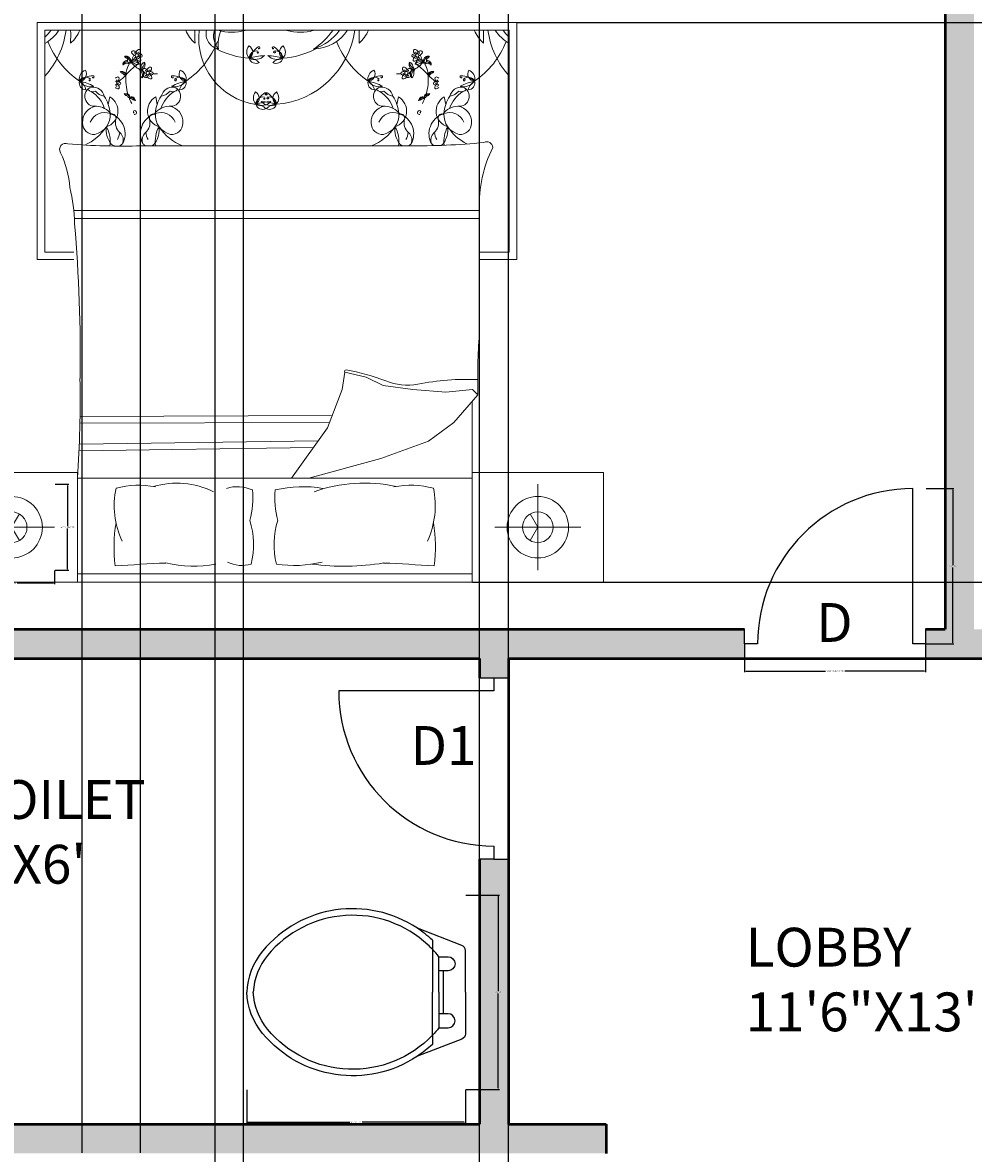
# Model space of a CAD drawing. Units: inches. Extents: x -15 to 420, y -514 to 86.
# Tile 5 of 8: x 65 to 212, y -251 to -76. Entities that reach past the tile are written whole.
import ezdxf

# ---------------------------------------------------------------- set-up
doc = ezdxf.new("R2010")
doc.units = ezdxf.units.IN
doc.header["$MEASUREMENT"] = 0
for name, color, linetype, lineweight in [('A-ANNO-DIMS', 2, 'Continuous', 18), ('A-ANNO-TEXT', 7, 'Continuous', 18), ('A-AREA-IDEN', 7, 'Continuous', 25), ('A-DOOR', 4, 'Continuous', 25), ('A-FLOR-FIXT', 9, 'Continuous', 25), ('A-FURN', 8, 'Continuous', 18), ('A-WALL', 7, 'Continuous', 50), ('A-WALL-PATT', 8, 'Continuous', 13)]:
    doc.layers.add(name, color=color, linetype=linetype, lineweight=lineweight)
doc.styles.get("Standard").update_dxf_attribs({"font": 'arial.ttf'})
doc.dimstyles.get("Standard").update_dxf_attribs({"dimtxt": 0.18, "dimasz": 0.18, "dimexe": 0.18, "dimexo": 0.0625, "dimgap": 0.09, "dimtad": 0, "dimtih": 1, "dimtoh": 1, "dimdec": 0, "dimzin": 0, "dimdsep": 46, "dimlunit": 3, "dimtxsty": 'Standard', "dimcen": 0.09, "dimadec": 0, "dimazin": 0, "dimtfac": 1, "dimtdec": 0, "dimtofl": 0, "dimtmove": 0, "dimatfit": 3, "dimfxl": 1, "dimtolj": 1, "dimtzin": 0, "dimarcsym": 0})

# ---------------------------------------------------------------- blocks, each defined once
blk = doc.blocks.new('DOOR-SWING-24IN')
for p, q in [((26, 0), (26, 24)), ((2, 0), (0, 0)), ((28, 0), (26, 0))]:
    blk.add_line(p, q)
blk.add_arc((26, 0), 24, 90, 180)
blk = doc.blocks.new('WC-PLAN')
for p, q in [((28.69, 20.98), (28.69, 19.56)), ((28.69, 19.56), (28.69, 12.91)), ((28.69, 6.26), (28.69, 12.91)), ((28.69, 6.26), (28.69, 4.85))]:
    blk.add_line(p, q)
for points in [[(26.37, 22.81, 0.383919), (2.44, 19.27, 0.163732), (0, 12.91, 0.359733)], [(28, 20.24, 0.431639), (3.21, 18.62, 0.162618), (1.01, 12.91, 0.470877)], [(28.69, 20.98, 0.040937), (26.37, 22.81, 0.163732)], [(33.8, 12.91), (33.8, 19.37, 0.31031), (33.26, 20.16), (26.37, 22.81, 0.209071)], [(28.69, 19.56, 0.014165), (28, 20.24, 0.162618)], [(29.71, 18.4, 0.022712), (28.69, 19.56, 0.162618)], [(29.71, 12.91), (29.71, 18.4, 0.022712)], [(29.71, 18.4), (31.12, 18.4, -1), (31.12, 16.24), (30.39, 16.24)], [(26.37, 3.02, -0.383919), (2.44, 6.56, -0.163732), (0, 12.91, -0.359733)], [(28.69, 6.26, -0.448546), (3.21, 7.2, -0.162618), (1.01, 12.91, -0.470877)], [(33.8, 12.91), (33.8, 6.46, -0.31031), (33.26, 5.67), (26.37, 3.02, -0.209071)], [(29.71, 12.91), (29.71, 7.43, -0.476108)], [(29.71, 7.43), (31.12, 7.43, 1), (31.12, 9.59), (30.39, 9.59)], [(29.71, 7.43, -0.022712), (28.69, 6.26, -0.162618)], [(28.69, 4.85, -0.040937), (26.37, 3.02, -0.163732)]]:
    blk.add_lwpolyline(points, format="xyb")
for points in [[(30.39, 16.24), (29.71, 16.24)], [(30.39, 9.59), (30.39, 16.24)], [(30.39, 9.59), (29.71, 9.59)]]:
    blk.add_lwpolyline(points)
blk = doc.blocks.new('BEDSIDE-LAMP-9-5IN')
for p, q in [((6.64, 13.29), (6.64, 0)), ((13.29, 6.64), (0, 6.64))]:
    blk.add_line(p, q)
for points in [[(6.64, 6.64), (7.83, 8.7)], [(6.64, 6.64), (7.83, 4.59)]]:
    blk.add_lwpolyline(points)
for radius in [4.75, 2.37]:
    blk.add_circle((6.64, 6.64), radius)
blk = doc.blocks.new('*D21')
at = {"layer": 'A-ANNO-DIMS', "color": 0, "lineweight": -2, "transparency": 16777216}
for p, q in [((176.92, -172.19), (176.92, -176.51)), ((204.92, -172.19), (204.92, -176.51)), ((177.1, -176.33), (189.41, -176.33)), ((204.74, -176.33), (192.44, -176.33))]:
    blk.add_line(p, q, dxfattribs=at)
at = {"layer": 'A-ANNO-DIMS', "color": 0, "transparency": 16777216}
for points in [[(177.1, -176.3), (177.1, -176.36), (176.92, -176.33)], [(204.74, -176.3), (204.74, -176.36), (204.92, -176.33)]]:
    blk.add_solid(points, dxfattribs=at)
at = {"layer": 'Defpoints', "color": 0, "transparency": 16777216}
for p in [(176.92, -172.13), (204.92, -172.13), (204.92, -176.33)]:
    blk.add_point(p, dxfattribs=at)
at = {"layer": 'A-ANNO-DIMS', "color": 0, "transparency": 16777216, "insert": (190.92, -176.33), "char_height": 0.18, "attachment_point": 5}
blk.add_mtext('\\A1;SWING DOOR 2\'-4" TYP.', dxfattribs=at)
blk = doc.blocks.new('*D22')
at = {"layer": 'A-ANNO-DIMS', "color": 0, "lineweight": -2, "transparency": 16777216}
for p, q in [((204.99, -148.13), (209.3, -148.13)), ((209.12, -148.31), (209.12, -159.95)), ((209.12, -171.95), (209.12, -160.31)), ((204.99, -172.13), (209.3, -172.13))]:
    blk.add_line(p, q, dxfattribs=at)
at = {"layer": 'A-ANNO-DIMS', "color": 0, "transparency": 16777216}
for points in [[(209.09, -148.31), (209.15, -148.31), (209.12, -148.13)], [(209.09, -171.95), (209.15, -171.95), (209.12, -172.13)]]:
    blk.add_solid(points, dxfattribs=at)
at = {"layer": 'Defpoints', "color": 0, "transparency": 16777216}
for p in [(204.92, -148.13), (209.12, -148.13), (204.92, -172.13)]:
    blk.add_point(p, dxfattribs=at)
at = {"layer": 'A-ANNO-DIMS', "color": 0, "transparency": 16777216, "insert": (209.12, -160.13), "char_height": 0.18, "attachment_point": 5}
blk.add_mtext('\\A1;2\'-0" TYP.', dxfattribs=at)
blk = doc.blocks.new('*D23')
at = {"layer": 'A-ANNO-DIMS', "color": 0, "lineweight": -2, "transparency": 16777216}
for p, q in [((99.95, -241.05), (99.95, -246.24)), ((133.75, -241.05), (133.75, -246.24)), ((100.13, -246.06), (115.89, -246.06)), ((133.57, -246.06), (117.81, -246.06))]:
    blk.add_line(p, q, dxfattribs=at)
at = {"layer": 'A-ANNO-DIMS', "color": 0, "transparency": 16777216}
for points in [[(100.13, -246.03), (100.13, -246.09), (99.95, -246.06)], [(133.57, -246.03), (133.57, -246.09), (133.75, -246.06)]]:
    blk.add_solid(points, dxfattribs=at)
at = {"layer": 'Defpoints', "color": 0, "transparency": 16777216}
for p in [(99.95, -240.99), (133.75, -240.99), (133.75, -246.06)]:
    blk.add_point(p, dxfattribs=at)
at = {"layer": 'A-ANNO-DIMS', "color": 0, "transparency": 16777216, "insert": (116.85, -246.06), "char_height": 0.18, "attachment_point": 5}
blk.add_mtext('\\A1;WC 2\'-10" TYP.', dxfattribs=at)
blk = doc.blocks.new('*D24')
at = {"layer": 'A-ANNO-DIMS', "color": 0, "lineweight": -2, "transparency": 16777216}
for p, q in [((133.81, -210.96), (139, -210.96)), ((138.82, -211.14), (138.82, -225.79)), ((138.82, -240.81), (138.82, -226.15)), ((133.81, -240.99), (139, -240.99))]:
    blk.add_line(p, q, dxfattribs=at)
at = {"layer": 'A-ANNO-DIMS', "color": 0, "transparency": 16777216}
for points in [[(138.79, -211.14), (138.85, -211.14), (138.82, -210.96)], [(138.79, -240.81), (138.85, -240.81), (138.82, -240.99)]]:
    blk.add_solid(points, dxfattribs=at)
at = {"layer": 'Defpoints', "color": 0, "transparency": 16777216}
for p in [(133.75, -210.96), (138.82, -210.96), (133.75, -240.99)]:
    blk.add_point(p, dxfattribs=at)
at = {"layer": 'A-ANNO-DIMS', "color": 0, "transparency": 16777216, "insert": (138.82, -225.97), "char_height": 0.18, "attachment_point": 5}
blk.add_mtext('\\A1;2\'-6" TYP.', dxfattribs=at)
blk = doc.blocks.new('*D35')
at = {"layer": 'A-ANNO-DIMS', "color": 0, "lineweight": -2, "transparency": 16777216}
for p, q in [((70.3, -147.46), (72.41, -147.46)), ((72.23, -147.64), (72.23, -153.92)), ((72.23, -160.57), (72.23, -154.29)), ((70.3, -160.75), (72.41, -160.75))]:
    blk.add_line(p, q, dxfattribs=at)
at = {"layer": 'A-ANNO-DIMS', "color": 0, "transparency": 16777216}
for points in [[(72.2, -147.64), (72.26, -147.64), (72.23, -147.46)], [(72.2, -160.57), (72.26, -160.57), (72.23, -160.75)]]:
    blk.add_solid(points, dxfattribs=at)
at = {"layer": 'Defpoints', "color": 0, "transparency": 16777216}
for p in [(70.24, -147.46), (72.23, -147.46), (70.24, -160.75)]:
    blk.add_point(p, dxfattribs=at)
at = {"layer": 'A-ANNO-DIMS', "color": 0, "transparency": 16777216, "insert": (72.23, -154.11), "char_height": 0.18, "attachment_point": 5}
blk.add_mtext('\\A1;LAMP 1\'-1 1/2" TYP.', dxfattribs=at)
blk = doc.blocks.new('*D36')
at = {"layer": 'A-ANNO-DIMS', "color": 0, "lineweight": -2, "transparency": 16777216}
for p, q in [((56.95, -160.81), (56.95, -162.92)), ((70.24, -160.81), (70.24, -162.92)), ((57.13, -162.74), (62.76, -162.74)), ((70.06, -162.74), (64.44, -162.74))]:
    blk.add_line(p, q, dxfattribs=at)
at = {"layer": 'A-ANNO-DIMS', "color": 0, "transparency": 16777216}
for points in [[(57.13, -162.71), (57.13, -162.77), (56.95, -162.74)], [(70.06, -162.71), (70.06, -162.77), (70.24, -162.74)]]:
    blk.add_solid(points, dxfattribs=at)
at = {"layer": 'Defpoints', "color": 0, "transparency": 16777216}
for p in [(56.95, -160.75), (70.24, -160.75), (70.24, -162.74)]:
    blk.add_point(p, dxfattribs=at)
at = {"layer": 'A-ANNO-DIMS', "color": 0, "transparency": 16777216, "insert": (63.6, -162.74), "char_height": 0.18, "attachment_point": 5}
blk.add_mtext('\\A1;1\'-1 1/2" TYP.', dxfattribs=at)
blk = doc.blocks.new('*D46')
at = {"layer": 'A-ANNO-DIMS', "color": 0, "lineweight": -2, "transparency": 16777216}
for p, q in [((74.51, -250.82), (74.51, 43.5)), ((74.69, 43.32), (78.68, 43.32)), ((83.33, 43.32), (79.34, 43.32)), ((83.51, -250.82), (83.51, 43.5))]:
    blk.add_line(p, q, dxfattribs=at)
at = {"layer": 'A-ANNO-DIMS', "color": 0, "transparency": 16777216}
for points in [[(74.69, 43.35), (74.69, 43.29), (74.51, 43.32)], [(83.33, 43.35), (83.33, 43.29), (83.51, 43.32)]]:
    blk.add_solid(points, dxfattribs=at)
at = {"layer": 'Defpoints', "color": 0, "transparency": 16777216}
for p in [(83.51, 43.32), (74.51, -250.88), (83.51, -250.88)]:
    blk.add_point(p, dxfattribs=at)
at = {"layer": 'A-ANNO-DIMS', "color": 0, "transparency": 16777216, "insert": (79.01, 43.32), "char_height": 0.18, "attachment_point": 5}
blk.add_mtext('\\A1;0\'-9"', dxfattribs=at)
blk = doc.blocks.new('*D48')
at = {"layer": 'A-ANNO-DIMS', "color": 0, "lineweight": -2, "transparency": 16777216}
for p, q in [((39.92, -250.82), (39.92, 43.5)), ((40.1, 43.32), (56.61, 43.32)), ((74.33, 43.32), (57.83, 43.32)), ((74.51, -250.82), (74.51, 43.5))]:
    blk.add_line(p, q, dxfattribs=at)
at = {"layer": 'A-ANNO-DIMS', "color": 0, "transparency": 16777216}
for points in [[(40.1, 43.35), (40.1, 43.29), (39.92, 43.32)], [(74.33, 43.35), (74.33, 43.29), (74.51, 43.32)]]:
    blk.add_solid(points, dxfattribs=at)
at = {"layer": 'Defpoints', "color": 0, "transparency": 16777216}
for p in [(74.51, 43.32), (39.92, -250.88), (74.51, -250.88)]:
    blk.add_point(p, dxfattribs=at)
at = {"layer": 'A-ANNO-DIMS', "color": 0, "transparency": 16777216, "insert": (57.22, 43.32), "char_height": 0.18, "attachment_point": 5}
blk.add_mtext('\\A1;2\'-10 1/2"', dxfattribs=at)
blk = doc.blocks.new('*D51')
at = {"layer": 'A-ANNO-DIMS', "color": 0, "lineweight": -2, "transparency": 16777216}
for p, q in [((135.92, -357.09), (135.92, 43.5)), ((136.1, 43.32), (137.64, 43.32)), ((140.24, 43.32), (138.71, 43.32)), ((140.42, -357.09), (140.42, 43.5))]:
    blk.add_line(p, q, dxfattribs=at)
at = {"layer": 'A-ANNO-DIMS', "color": 0, "transparency": 16777216}
for points in [[(136.1, 43.35), (136.1, 43.29), (135.92, 43.32)], [(140.24, 43.35), (140.24, 43.29), (140.42, 43.32)]]:
    blk.add_solid(points, dxfattribs=at)
at = {"layer": 'Defpoints', "color": 0, "transparency": 16777216}
for p in [(140.42, 43.32), (135.92, -357.15), (140.42, -357.15)]:
    blk.add_point(p, dxfattribs=at)
at = {"layer": 'A-ANNO-DIMS', "color": 0, "transparency": 16777216, "insert": (138.17, 43.32), "char_height": 0.18, "attachment_point": 5}
blk.add_mtext('\\A1;0\'-4 1/2"', dxfattribs=at)
blk = doc.blocks.new('*D58')
at = {"layer": 'A-ANNO-DIMS', "color": 0, "lineweight": -2, "transparency": 16777216}
for p, q in [((95.06, -434.9), (95.06, 43.5)), ((95.24, 43.32), (96.7, 43.32)), ((99.24, 43.32), (97.78, 43.32)), ((99.42, -434.9), (99.42, 43.5))]:
    blk.add_line(p, q, dxfattribs=at)
at = {"layer": 'A-ANNO-DIMS', "color": 0, "transparency": 16777216}
for points in [[(95.24, 43.35), (95.24, 43.29), (95.06, 43.32)], [(99.24, 43.35), (99.24, 43.29), (99.42, 43.32)]]:
    blk.add_solid(points, dxfattribs=at)
at = {"layer": 'Defpoints', "color": 0, "transparency": 16777216}
for p in [(99.42, 43.32), (95.06, -434.96), (99.42, -434.96)]:
    blk.add_point(p, dxfattribs=at)
at = {"layer": 'A-ANNO-DIMS', "color": 0, "transparency": 16777216, "insert": (97.24, 43.32), "char_height": 0.18, "attachment_point": 5}
blk.add_mtext('\\A1;0\'-4 1/2"', dxfattribs=at)
blk = doc.blocks.new('*D69')
at = {"layer": 'A-ANNO-DIMS', "color": 0, "lineweight": -2, "transparency": 16777216}
for p, q in [((141.76, -76.1), (419.8, -76.1)), ((419.62, -76.28), (419.62, -119.16)), ((419.62, -162.4), (419.62, -119.53)), ((134.84, -162.58), (419.8, -162.58))]:
    blk.add_line(p, q, dxfattribs=at)
at = {"layer": 'A-ANNO-DIMS', "color": 0, "transparency": 16777216}
for points in [[(419.59, -76.28), (419.65, -76.28), (419.62, -76.1)], [(419.59, -162.4), (419.65, -162.4), (419.62, -162.58)]]:
    blk.add_solid(points, dxfattribs=at)
at = {"layer": 'Defpoints', "color": 0, "transparency": 16777216}
for p in [(141.69, -76.1), (134.78, -162.58), (419.62, -162.58)]:
    blk.add_point(p, dxfattribs=at)
at = {"layer": 'A-ANNO-DIMS', "color": 0, "transparency": 16777216, "insert": (419.62, -119.34), "char_height": 0.18, "attachment_point": 5}
blk.add_mtext('\\A1;7\'-2 1/2"', dxfattribs=at)

msp = doc.modelspace()

# ---------------------------------------------------------------- hatches: boundary and pattern name
at = {"layer": 'A-WALL-PATT'}
h = msp.add_hatch(color=256, dxfattribs=at)
h.dxf.hatch_style = 1
h.paths.add_polyline_path([(266.67, -454.88), (240.92, -454.88), (240.92, -330.38), (236.42, -330.38), (236.42, -454.88), (218.42, -454.88), (218.42, -463.88), (266.67, -463.88)])
h.paths.add_polyline_path([(158.42, -454.88), (140.42, -454.88), (140.42, -394.88), (135.92, -394.88), (135.92, -454.88), (39.92, -454.88), (39.92, -412.88), (30.92, -412.88), (30.92, -463.88), (158.42, -463.88)])
h.paths.add_polyline_path([(39.92, -334.88), (135.92, -334.88), (135.92, -357.15), (140.42, -357.15), (140.42, -334.88), (173.95, -334.88), (173.95, -330.38), (39.92, -330.38), (39.92, -250.88), (155.51, -250.88), (155.51, -246.38), (140.42, -246.38), (140.42, -205.38), (138.17, -205.38), (135.92, -205.38), (135.92, -246.38), (39.92, -246.38), (39.92, -222.38), (30.92, -222.38), (30.92, -376.88), (39.92, -376.88)])
h.paths.add_polyline_path([(389.42, -382.88), (380.42, -382.88), (380.42, -454.88), (380.42, -463.88), (389.42, -463.88)])
h.paths.add_polyline_path([(352.42, -459.38), (352.42, -454.88), (326.67, -454.88), (326.67, -463.88), (352.42, -463.88)])
h.paths.add_polyline_path([(176.92, -169.88), (39.92, -169.88), (39.92, -112.88), (30.92, -112.88), (30.92, -198.38), (39.92, -198.38), (39.92, -174.38), (135.92, -174.38), (135.92, -177.38), (140.42, -177.38), (140.42, -174.38), (176.92, -174.38), (176.92, -172.13)])
h.paths.add_polyline_path([(39.92, 4.12), (93.92, 4.12), (93.92, 13.12), (30.92, 13.12), (30.92, -52.88), (39.92, -52.88)])
h.paths.add_polyline_path([(266.42, 13.12), (153.92, 13.12), (153.92, 4.12), (207.92, 4.12), (207.92, -169.88), (204.92, -169.88), (204.92, -174.38), (215.42, -174.38), (215.42, -169.88), (212.42, -169.88), (212.42, 4.12), (266.42, 4.12)])
h.paths.add_polyline_path([(389.42, 13.12), (326.42, 13.12), (326.42, 4.12), (380.42, 4.12), (380.42, -52.88), (389.42, -52.88)])
h.paths.add_polyline_path([(389.42, -112.88), (380.42, -112.88), (380.42, -169.88), (377.42, -169.88), (377.42, -174.38), (380.42, -174.38), (380.42, -198.38), (389.42, -198.38)])
h.paths.add_polyline_path([(349.42, -172.13), (349.42, -169.88), (243.42, -169.88), (243.42, -172.13), (243.42, -174.38), (279.92, -174.38), (279.92, -250.88), (380.42, -250.88), (380.42, -322.88), (389.42, -322.88), (389.42, -222.38), (380.42, -222.38), (380.42, -246.38), (284.42, -246.38), (284.42, -174.38), (349.42, -174.38)])

# ---------------------------------------------------------------- linework, layer by layer
at = {"layer": 'A-DOOR'}
for p, q in [((176.92, -172.13), (176.92, -169.88)), ((204.92, -169.88), (204.92, -174.38)), ((176.92, -172.13), (176.92, -174.38)), ((135.92, -177.38), (140.42, -177.38)), ((138.17, -205.38), (135.92, -205.38)), ((138.17, -205.38), (140.42, -205.38))]:
    msp.add_line(p, q, dxfattribs=at)
at = {"layer": 'A-FURN'}
for p, q in [((67.56, -76.1), (141.69, -76.1)), ((67.56, -112.73), (67.56, -76.1)), ((141.69, -76.1), (141.69, -112.73)), ((68.74, -77.28), (68.74, -111.56)), ((140.51, -77.28), (68.74, -77.28)), ((140.51, -111.56), (140.51, -77.28)), ((78.76, -87.59), (78.53, -88.74)), ((85.86, -87.59), (86.09, -88.74)), ((123.39, -87.59), (123.16, -88.74)), ((130.49, -87.59), (130.72, -88.74)), ((83.63, -95.14), (124.91, -95.14)), ((73.21, -105.12), (135.95, -105.12)), ((73.3, -106.39), (135.95, -106.39)), ((68.74, -111.56), (73.22, -111.56)), ((135.94, -111.56), (140.51, -111.56)), ((73.2, -112.73), (67.56, -112.73)), ((141.69, -112.73), (135.94, -112.73)), ((114.68, -132.79), (115.09, -130.11)), ((115.09, -130.11), (118.39, -130.93)), ((118.39, -130.93), (121.06, -132.17)), ((112.41, -138.76), (114.68, -132.79)), ((121.06, -132.17), (125.6, -132.79)), ((125.6, -132.79), (130.74, -133.2)), ((130.74, -133.2), (134.86, -132.79)), ((134.86, -132.79), (135.69, -133.61)), ((135.69, -133.61), (131.98, -137.93)), ((134.78, -162.58), (134.78, -134.67)), ((74.13, -137), (113.14, -136.84)), ((74.13, -138.04), (112.74, -137.89)), ((131.98, -137.93), (128.07, -140.81)), ((106.84, -146.51), (112.41, -138.76)), ((74.08, -141.24), (111, -140.72)), ((128.07, -140.81), (120.65, -143.49)), ((74.04, -142.29), (110.24, -141.78)), ((120.65, -143.49), (109.56, -146.51)), ((134.78, -146.51), (73.77, -146.51)), ((73.77, -161.28), (134.78, -161.28)), ((155.11, -162.58), (53.43, -162.58))]:
    msp.add_line(p, q, dxfattribs=at)
for points in [[(135.9, -124.3, 0.001242), (135.95, -105, -0.127202), (137.99, -95.39)], [(73.33, -107.19, 0.056112), (72.59, -101.6, 0.095341), (71.16, -96.21)], [(79.61, -160.05, -0.074897), (79.73, -153.41, 0.472817)], [(100.41, -153.03, -0.14099), (100.61, -159.81, -0.235245)], [(104.75, -153.03, 0.14099), (104.54, -159.81, 0.235245)], [(128.94, -160.05, 0.074897), (128.81, -153.41, -0.472817)]]:
    msp.add_lwpolyline(points, format="xyb", dxfattribs=at)
for points in [[(73.77, -162.58), (73.77, -145.63), (53.43, -145.63), (53.43, -162.58)], [(134.78, -145.63), (155.11, -145.63), (155.11, -162.58)]]:
    msp.add_lwpolyline(points, dxfattribs=at)
for centre in [(82.94, -81.18), (126.31, -81.18), (84.63, -83.91), (124.62, -83.91)]:
    msp.add_circle(centre, 0.259, dxfattribs=at)
for centre, radius, start, end in [((65.51, -73.71), 6.47, 299.8884, 326.5383), ((63.19, -72.51), 8.06, 313.5186, 323.6964), ((58.85, -75.49), 13.28, 318.1144, 352.255), ((69.14, -75.21), 5.4, 311.0454, 337.4453), ((54.35, -78.11), 18.37, 356.3481, 2.5919), ((95.49, -75.21), 5.4, 202.5547, 228.9546), ((110.28, -78.11), 18.37, 177.4081, 183.6519), ((102.81, -78.56), 10.28, 172.8636, 261.8197), ((96.03, -77.84), 2.38, 166.3898, 259.0739), ((97.82, -78.17), 3.01, 162.8609, 221.9049), ((97.65, -70.3), 7.3, 252.9798, 286.4569), ((101.48, -79.5), 5.95, 158.117, 186.6195), ((100.54, -66.54), 10.8, 264.3643, 265.6213), ((106.23, -59.14), 19.29, 250.0972, 250.2783), ((103.48, -75.49), 13.28, 274.4623, 352.255), ((108.21, -70.3), 7.3, 253.5431, 287.0202), ((105.32, -66.54), 10.8, 274.3787, 275.6357), ((99.63, -59.14), 19.29, 289.7217, 289.9028), ((110.14, -73.71), 6.47, 271.272, 326.5383), ((103.58, -70.24), 11.99, 304.0123, 324.053), ((107.81, -72.51), 8.06, 287.8504, 323.6964), ((98.98, -78.11), 18.37, 356.3481, 2.5919), ((113.77, -75.21), 5.4, 311.0454, 337.4453), ((140.12, -75.21), 5.4, 202.5547, 228.9546), ((154.9, -78.11), 18.37, 177.4081, 183.6519), ((150.4, -75.49), 13.28, 187.745, 221.8856), ((143.74, -73.71), 6.47, 213.4617, 240.1116), ((146.07, -72.51), 8.06, 216.3036, 226.4814), ((81.57, -74.18), 13.28, 201.4092, 235.6135), ((83.29, -80.7), 0.428, 100.9597, 208.7804), ((83.33, -80.44), 0.199, 4.947, 127.5263), ((83.05, -74.18), 13.28, 304.3865, 338.5908), ((101.37, -68.38), 13.28, 242.5854, 265.5377), ((101.42, -80.63), 1.47, 140.8855, 222.2127), ((99.75, -80.67), 1.11, 301.6373, 61.4609), ((103.51, -82.71), 3.36, 121.989, 161.0841), ((101.82, -80), 0.165, 288.4408, 121.989), ((101.84, -80.08), 0.0801, 171.9833, 288.4408), ((104.05, -80), 0.165, 58.011, 251.5592), ((104.02, -80.08), 0.0801, 251.5592, 8.0167), ((102.35, -82.71), 3.36, 18.9159, 58.011), ((106.11, -80.67), 1.11, 118.5391, 238.3627), ((104.44, -80.63), 1.47, 317.7873, 39.1145), ((104.5, -68.38), 13.28, 274.4623, 297.4146), ((126.2, -74.18), 13.28, 201.4092, 235.6135), ((125.92, -80.44), 0.199, 52.4737, 175.053), ((125.96, -80.7), 0.428, 331.2196, 79.0403), ((127.68, -74.18), 13.28, 304.3865, 338.5908), ((81.55, -82.92), 0.783, 92.3172, 160.5201), ((81.46, -82.62), 0.674, 82.6008, 147.1845), ((81.27, -81.55), 0.289, 55.6077, 145.6462), ((81.07, -82.17), 0.783, 21.7087, 93.0299), ((76.95, -87.76), 7.57, 53.6254, 57.3216), ((81.31, -81.98), 0.674, 342.8042, 79.6943), ((81.25, -81.91), 0.299, 338.2452, 53.6254), ((81.74, -82.1), 0.226, 158.2452, 340.6395), ((81.74, -82.27), 0.226, 225.7354, 48.1297), ((85.99, -80.22), 4.51, 201.7087, 206.2181), ((82.4, -83.3), 1.18, 40.9365, 112.7695), ((85.46, -84.56), 4.22, 137.5083, 145.9967), ((82.52, -82.62), 0.718, 61.1838, 141.6792), ((82.39, -80.69), 0.257, 134.3732, 211.9501), ((82.87, -80.39), 0.816, 211.9501, 255.2442), ((82.41, -80.98), 0.511, 8.5614, 112.5914), ((82.65, -81.54), 0.353, 88.5719, 233.8954), ((82.61, -81.63), 0.254, 228.2946, 6.2474), ((82.56, -80.96), 0.172, 352.868, 97.094), ((82.38, -81.33), 0.356, 298.8493, 359.9355), ((82.46, -81.64), 0.407, 4.2123, 48.1587), ((82.47, -82.75), 0.858, 15.6484, 62.2957), ((83.3, -81.58), 0.432, 183.635, 258.4363), ((83.24, -81.42), 0.247, 178.1325, 268.8919), ((83.75, -81.27), 0.786, 132.3896, 156.5724), ((83.41, -81.37), 0.424, 42.3208, 130.2111), ((83.5, -80.92), 0.535, 226.3462, 279.6513), ((82.93, -80.47), 0.602, 291.6382, 4.947), ((82.95, -81.92), 0.623, 7.4968, 71.2737), ((83.4, -80.37), 0.848, 254.2829, 276.9148), ((83.37, -81.89), 0.2, 215.0752, 14.7644), ((83.56, -81.23), 0.223, 279.6513, 42.3208), ((101.42, -81.58), 1.09, 76.148, 182.2415), ((103.11, -90.48), 9.29, 92.7418, 107.407), ((101.2, -79.71), 2.1, 245.6899, 314.4589), ((100.27, -83.89), 2.27, 44.6273, 88.5415), ((101.39, -81.31), 1.1, 196.1963, 296.9726), ((101.66, -80.72), 0.0866, 140.1909, 76.0209), ((102.75, -90.48), 9.29, 72.593, 87.2582), ((104.67, -79.71), 2.1, 225.5411, 294.3101), ((105.59, -83.89), 2.27, 91.4585, 135.3727), ((104.47, -81.31), 1.1, 243.0274, 343.8037), ((104.22, -80.66), 0.144, 103.852, 39.9245), ((104.45, -81.58), 1.09, 357.7585, 103.852), ((125.7, -81.23), 0.223, 137.6792, 260.3487), ((125.84, -81.37), 0.424, 49.7889, 137.6792), ((125.75, -80.92), 0.535, 260.3487, 313.6538), ((126.3, -81.92), 0.623, 108.7263, 172.5032), ((125.88, -81.89), 0.2, 165.2356, 324.9248), ((126.32, -80.47), 0.602, 175.053, 248.3618), ((125.85, -80.37), 0.848, 263.0852, 285.7171), ((126.79, -82.75), 0.858, 117.7043, 164.3516), ((126.85, -83.3), 1.18, 67.2305, 139.0635), ((126.01, -81.42), 0.247, 271.1081, 1.8675), ((125.5, -81.27), 0.786, 23.4276, 47.6104), ((125.96, -81.58), 0.432, 281.5637, 356.365), ((126.84, -80.98), 0.511, 67.4086, 171.4386), ((126.64, -81.63), 0.254, 173.7526, 311.7054), ((126.79, -81.64), 0.407, 131.8413, 175.7877), ((126.73, -82.62), 0.718, 38.3208, 118.8162), ((126.88, -81.33), 0.356, 180.0645, 241.1507), ((126.7, -80.96), 0.172, 82.906, 187.132), ((126.38, -80.39), 0.816, 284.7558, 328.0499), ((126.6, -81.54), 0.353, 306.1046, 91.4281), ((123.8, -84.56), 4.22, 34.0033, 42.4917), ((126.86, -80.69), 0.257, 328.0499, 45.6268), ((127.94, -81.98), 0.674, 100.3057, 197.1958), ((127.51, -82.27), 0.226, 131.8703, 314.2646), ((127.51, -82.1), 0.226, 199.3605, 21.7548), ((123.26, -80.22), 4.51, 333.7819, 338.2913), ((128.18, -82.17), 0.783, 86.9701, 158.2913), ((128, -81.91), 0.299, 126.3746, 201.7548), ((127.79, -82.62), 0.674, 32.8155, 97.3992), ((127.7, -82.92), 0.783, 19.4799, 87.6828), ((127.98, -81.55), 0.289, 34.3538, 124.3923), ((132.31, -87.76), 7.57, 122.6784, 126.3746), ((75.51, -84.82), 1.47, 110.9613, 192.2885), ((74.04, -84.03), 1.11, 271.7131, 31.5367), ((80.48, -86.53), 2.87, 82.8698, 91.6736), ((80.87, -83.44), 0.534, 205.5379, 258.6744), ((80.11, -85.25), 1.61, 59.344, 79.7412), ((81.05, -82.5), 0.289, 123.0979, 213.1364), ((85.13, -88.87), 7.57, 121.1156, 124.8118), ((80.76, -84.17), 0.488, 355.7131, 81.6568), ((80.49, -84.6), 0.852, 27.3659, 59.344), ((81.38, -82.65), 0.299, 45.7354, 121.1156), ((85.46, -84.56), 4.22, 150.7959, 175.244), ((91.53, -93.55), 13.89, 127.8256, 137.7588), ((82.01, -82.9), 0.695, 49.3812, 95.5456), ((85.89, -78.95), 5.06, 220.182, 239.456), ((83.01, -81.74), 0.835, 229.3812, 289.9959), ((82.96, -82.2), 1.18, 287.889, 359.722), ((82.92, -82.75), 0.695, 305.1128, 351.2773), ((83.28, -84.03), 0.718, 3.8774, 87.1501), ((82.77, -83.75), 0.695, 352.0748, 38.2393), ((82.65, -84.29), 1.18, 343.6301, 55.4631), ((84.29, -83.96), 0.835, 172.0748, 232.6895), ((83.49, -82.63), 0.718, 271.4625, 339.4747), ((84.43, -82.98), 0.835, 110.6625, 171.2773), ((84.09, -83.42), 0.257, 134.3732, 211.9501), ((85.89, -78.95), 5.06, 246.1523, 246.9499), ((84.56, -83.12), 0.816, 211.9501, 255.2442), ((84.11, -83.71), 0.511, 8.5614, 112.5914), ((83.36, -82.56), 0.858, 338.3627, 25.0101), ((84.25, -83.69), 0.172, 352.868, 97.094), ((84.99, -83.43), 0.428, 100.9597, 208.7804), ((85.45, -84), 0.786, 132.3896, 156.5724), ((85.1, -84.1), 0.424, 42.3208, 130.2111), ((84.62, -83.2), 0.602, 291.6382, 4.947), ((85.03, -83.17), 0.199, 4.947, 127.5263), ((85.25, -83.96), 0.223, 279.6513, 42.3208), ((90.59, -84.03), 1.11, 148.4633, 268.2869), ((89.11, -84.82), 1.47, 347.7115, 69.0387), ((120.14, -84.82), 1.47, 110.9613, 192.2885), ((118.67, -84.03), 1.11, 271.7131, 31.5367), ((124, -83.96), 0.223, 137.6792, 260.3487), ((124.15, -84.1), 0.424, 49.7889, 137.6792), ((124.23, -83.17), 0.199, 52.4737, 175.053), ((124.63, -83.2), 0.602, 175.053, 248.3618), ((123.8, -84), 0.786, 23.4276, 47.6104), ((124.27, -83.43), 0.428, 331.2196, 79.0403), ((125.15, -83.71), 0.511, 67.4086, 171.4386), ((125, -83.69), 0.172, 82.906, 187.132), ((124.69, -83.12), 0.816, 284.7558, 328.0499), ((125.89, -82.56), 0.858, 154.9899, 201.6373), ((125.77, -82.63), 0.718, 200.5253, 268.5375), ((126.3, -82.2), 1.18, 180.278, 252.111), ((124.82, -82.98), 0.835, 8.7227, 69.3375), ((125.97, -84.03), 0.718, 92.8499, 176.1226), ((125.16, -83.42), 0.257, 328.0499, 45.6268), ((123.36, -78.95), 5.06, 293.0501, 293.8477), ((126.6, -84.29), 1.18, 124.5369, 196.3699), ((124.96, -83.96), 0.835, 307.3105, 7.9252), ((126.33, -82.75), 0.695, 188.7227, 234.8872), ((126.48, -83.75), 0.695, 141.7607, 187.9252), ((123.36, -78.95), 5.06, 300.544, 319.818), ((126.25, -81.74), 0.835, 250.0041, 310.6188), ((117.72, -93.55), 13.89, 42.2412, 52.1744), ((127.24, -82.9), 0.695, 84.4544, 130.6188), ((123.8, -84.56), 4.22, 4.756, 29.2041), ((127.88, -82.65), 0.299, 58.8844, 134.2646), ((128.49, -84.17), 0.488, 98.3432, 184.2869), ((128.76, -84.6), 0.852, 120.656, 152.6341), ((124.12, -88.87), 7.57, 55.1882, 58.8844), ((129.15, -85.25), 1.61, 100.2588, 120.656), ((128.2, -82.5), 0.289, 326.8636, 56.9021), ((128.78, -86.53), 2.87, 88.3264, 97.1302), ((128.38, -83.44), 0.534, 281.3256, 334.4621), ((135.22, -84.03), 1.11, 148.4633, 268.2869), ((133.74, -84.82), 1.47, 347.7115, 69.0387), ((75.14, -85.4), 1.1, 166.272, 267.0484), ((76.28, -87.67), 3.36, 92.0648, 131.1598), ((75.03, -85.64), 1.09, 46.2238, 152.3173), ((72.06, -94.21), 9.29, 62.8176, 77.4827), ((75.77, -83.91), 2.1, 215.7657, 284.5347), ((72.89, -87.07), 2.27, 14.7031, 58.6173), ((75.67, -85.02), 0.0866, 110.2667, 46.2271), ((76.15, -84.56), 0.0801, 142.0591, 258.5166), ((76.17, -84.48), 0.165, 258.5166, 92.0648), ((79.97, -84.97), 0.428, 100.9597, 142.2379), ((79.61, -85.45), 0.259, 273.2768, 86.7232), ((80.43, -85.54), 0.786, 132.3896, 156.5724), ((80.08, -85.64), 0.424, 42.3208, 130.2111), ((80.18, -85.19), 0.535, 226.3462, 279.6513), ((79.62, -86.19), 0.623, 7.4968, 71.2737), ((79.6, -84.74), 0.602, 291.6382, 4.947), ((80.08, -84.64), 0.848, 254.2829, 276.9148), ((80.01, -84.7), 0.199, 4.947, 127.5263), ((74.21, -77.6), 9.65, 307.9541, 316.8459), ((80.23, -85.5), 0.223, 279.6513, 42.3208), ((79.76, -85.24), 1.63, 43.6929, 51.7899), ((81.13, -84.04), 0.207, 202.5583, 304.2343), ((89.65, -84.77), 8.42, 176.1723, 196.4158), ((83.14, -84.05), 0.858, 318.342, 4.9894), ((84.35, -84.27), 0.353, 88.5719, 233.8954), ((84.31, -84.36), 0.254, 228.2946, 6.2474), ((84.07, -84.06), 0.356, 298.8493, 359.9355), ((84.15, -84.37), 0.407, 4.2123, 48.1587), ((84.99, -84.31), 0.432, 183.635, 258.4363), ((84.93, -84.15), 0.247, 178.1325, 268.8919), ((85.2, -83.65), 0.535, 226.3462, 279.6513), ((84.64, -84.65), 0.623, 7.4968, 71.2737), ((85.1, -83.1), 0.848, 254.2829, 276.9148), ((85.07, -84.62), 0.2, 215.0752, 14.7644), ((85.89, -78.95), 5.06, 265.2415, 272.8929), ((88.46, -84.48), 0.165, 87.9352, 281.4834), ((88.85, -83.91), 2.1, 255.4653, 324.2343), ((92.57, -94.21), 9.29, 102.5173, 117.1824), ((88.34, -87.67), 3.36, 48.8402, 87.9352), ((88.47, -84.56), 0.0801, 281.4834, 37.9409), ((88.94, -84.96), 0.144, 133.7762, 69.7183), ((89.59, -85.64), 1.09, 27.6827, 133.7762), ((89.48, -85.4), 1.1, 272.9516, 13.728), ((91.73, -87.07), 2.27, 121.3827, 165.2969), ((119.77, -85.4), 1.1, 166.272, 267.0484), ((120.91, -87.67), 3.36, 92.0648, 131.1598), ((119.66, -85.64), 1.09, 46.2238, 152.3173), ((117.52, -87.07), 2.27, 14.7031, 58.6173), ((120.4, -83.91), 2.1, 215.7657, 284.5347), ((116.69, -94.21), 9.29, 62.8176, 77.4827), ((120.3, -85.02), 0.0866, 110.2667, 46.2271), ((120.78, -84.56), 0.0801, 142.0591, 258.5166), ((120.79, -84.48), 0.165, 258.5166, 92.0648), ((123.36, -78.95), 5.06, 267.1071, 274.7585), ((124.05, -83.65), 0.535, 260.3487, 313.6538), ((124.18, -84.62), 0.2, 165.2356, 324.9248), ((124.61, -84.65), 0.623, 108.7263, 172.5032), ((124.16, -83.1), 0.848, 263.0852, 285.7171), ((124.32, -84.15), 0.247, 271.1081, 1.8675), ((124.26, -84.31), 0.432, 281.5637, 356.365), ((125.1, -84.37), 0.407, 131.8413, 175.7877), ((124.94, -84.36), 0.254, 173.7526, 311.7054), ((125.18, -84.06), 0.356, 180.0645, 241.1507), ((124.91, -84.27), 0.353, 306.1046, 91.4281), ((126.11, -84.05), 0.858, 175.0106, 221.658), ((119.6, -84.77), 8.42, 343.5842, 3.8277), ((128.12, -84.04), 0.207, 235.7657, 337.4417), ((135.05, -77.6), 9.65, 223.1541, 232.0459), ((129.49, -85.24), 1.63, 128.2101, 136.3071), ((129.02, -85.5), 0.223, 137.6792, 260.3487), ((129.17, -85.64), 0.424, 49.7889, 137.6792), ((129.08, -85.19), 0.535, 260.3487, 313.6538), ((129.63, -86.19), 0.623, 108.7263, 172.5032), ((129.25, -84.7), 0.199, 52.4737, 175.053), ((129.65, -84.74), 0.602, 175.053, 248.3618), ((129.18, -84.64), 0.848, 263.0852, 285.7171), ((128.83, -85.54), 0.786, 23.4276, 47.6104), ((129.29, -84.97), 0.428, 37.7621, 79.0403), ((129.64, -85.45), 0.259, 93.2768, 266.7232), ((133.09, -84.48), 0.165, 87.9352, 281.4834), ((137.2, -94.21), 9.29, 102.5173, 117.1824), ((133.48, -83.91), 2.1, 255.4653, 324.2343), ((132.97, -87.67), 3.36, 48.8402, 87.9352), ((133.1, -84.56), 0.0801, 281.4834, 37.9409), ((133.57, -84.96), 0.144, 133.7762, 69.7183), ((134.22, -85.64), 1.09, 27.6827, 133.7762), ((136.36, -87.07), 2.27, 121.3827, 165.2969), ((134.11, -85.4), 1.1, 272.9516, 13.728), ((76.43, -87.51), 1.53, 109.1312, 279.736), ((76.12, -85.86), 0.935, 216.7319, 296.0245), ((73.41, -90.87), 4.8, 18.2955, 58.7386), ((76.07, -87.97), 1.91, 15.6955, 94.031), ((78.12, -85.43), 2.03, 218.4175, 263.8338), ((79.97, -85.85), 0.432, 217.3642, 258.4363), ((79.91, -85.69), 0.247, 178.1325, 268.8919), ((80.05, -86.16), 0.2, 215.0752, 14.7644), ((81.08, -89.96), 2.87, 82.8698, 91.6736), ((81.48, -86.86), 0.534, 205.5379, 258.6744), ((80.71, -88.67), 1.61, 59.344, 79.7412), ((80.37, -88.67), 1.63, 43.6929, 51.7899), ((81.37, -87.59), 0.488, 355.7131, 81.6568), ((81.1, -88.02), 0.852, 27.3659, 59.344), ((91.22, -90.87), 4.8, 121.2614, 161.7045), ((88.56, -87.97), 1.91, 85.969, 164.3045), ((86.5, -85.43), 2.03, 276.1662, 321.5825), ((88.19, -87.51), 1.53, 260.264, 70.8688), ((88.5, -85.86), 0.935, 243.9755, 323.2681), ((102.44, -87.74), 1.47, 140.8855, 222.2127), ((100.77, -87.79), 1.11, 301.6373, 61.4609), ((104.53, -89.82), 3.36, 121.989, 161.0841), ((102.83, -87.11), 0.165, 288.4408, 121.989), ((102.86, -87.19), 0.0801, 171.9833, 288.4408), ((103.03, -87.11), 0.165, 58.011, 251.5592), ((103, -87.19), 0.0801, 251.5592, 8.0167), ((101.34, -89.82), 3.36, 18.9159, 58.011), ((105.1, -87.79), 1.11, 118.5391, 238.3627), ((103.42, -87.74), 1.47, 317.7873, 39.1145), ((121.06, -87.51), 1.53, 109.1312, 279.736), ((120.75, -85.86), 0.935, 216.7319, 296.0245), ((118.04, -90.87), 4.8, 18.2955, 58.7386), ((120.7, -87.97), 1.91, 15.6955, 94.031), ((122.75, -85.43), 2.03, 218.4175, 263.8338), ((127.88, -87.59), 0.488, 98.3432, 184.2869), ((128.15, -88.02), 0.852, 120.656, 152.6341), ((128.89, -88.67), 1.63, 128.2101, 136.3071), ((128.54, -88.67), 1.61, 100.2588, 120.656), ((128.17, -89.96), 2.87, 88.3264, 97.1302), ((127.77, -86.86), 0.534, 281.3256, 334.4621), ((129.2, -86.16), 0.2, 165.2356, 324.9248), ((129.34, -85.69), 0.247, 271.1081, 1.8675), ((129.28, -85.85), 0.432, 281.5637, 322.6358), ((135.85, -90.87), 4.8, 121.2614, 161.7045), ((133.19, -87.97), 1.91, 85.969, 164.3045), ((131.13, -85.43), 2.03, 276.1662, 321.5825), ((132.82, -87.51), 1.53, 260.264, 70.8688), ((133.13, -85.86), 0.935, 243.9755, 323.2681), ((76.99, -91.42), 2.43, 97.1143, 185.0551), ((76.57, -91.96), 2.95, 35.9599, 87.6409), ((73.36, -90.48), 5.46, 3.4924, 33.7117), ((77.5, -89.78), 2.53, 286.8663, 60.0915), ((81.74, -87.46), 0.207, 202.5583, 304.2343), ((89.65, -84.77), 8.42, 200.1059, 206.9968), ((82.12, -88.04), 0.488, 36.5232, 122.4668), ((81.87, -88.48), 0.852, 58.836, 90.8141), ((82.06, -87.65), 0.207, 173.9457, 275.6216), ((81.64, -89.43), 1.63, 66.3901, 74.4871), ((82.71, -87.59), 0.534, 219.5056, 272.6421), ((81.48, -89.13), 1.61, 38.4388, 58.836), ((80.17, -89.41), 2.87, 26.5064, 35.3102), ((87.13, -89.78), 2.53, 119.9085, 253.1337), ((88.05, -91.96), 2.95, 92.3591, 144.0401), ((91.26, -90.48), 5.46, 146.2883, 176.5076), ((87.63, -91.42), 2.43, 354.9449, 82.8857), ((102.43, -88.69), 1.09, 76.148, 182.2415), ((102.21, -86.82), 2.1, 245.6899, 314.4589), ((104.13, -97.6), 9.29, 92.7418, 107.407), ((102.41, -88.42), 1.1, 196.1963, 296.9726), ((101.29, -91), 2.27, 44.6273, 88.5415), ((103.65, -86.82), 2.1, 225.5411, 294.3101), ((101.73, -97.6), 9.29, 72.593, 87.2582), ((102.67, -87.83), 0.0866, 140.1909, 76.0209), ((103.46, -88.42), 1.1, 243.0274, 343.8037), ((104.57, -91), 2.27, 91.4585, 135.3727), ((103.2, -87.77), 0.144, 103.852, 39.9245), ((103.43, -88.69), 1.09, 357.7585, 103.852), ((121.62, -91.42), 2.43, 97.1143, 185.0551), ((121.2, -91.96), 2.95, 35.9599, 87.6409), ((117.99, -90.48), 5.46, 3.4924, 33.7117), ((122.13, -89.78), 2.53, 286.8663, 60.0915), ((127.78, -89.13), 1.61, 121.164, 141.5612), ((129.08, -89.41), 2.87, 144.6898, 153.4936), ((126.54, -87.59), 0.534, 267.3579, 320.4944), ((127.14, -88.04), 0.488, 57.5332, 143.4768), ((127.39, -88.48), 0.852, 89.1859, 121.164), ((127.61, -89.43), 1.63, 105.5129, 113.6099), ((119.6, -84.77), 8.42, 333.0032, 339.8941), ((127.19, -87.65), 0.207, 264.3784, 6.0543), ((127.51, -87.46), 0.207, 235.7657, 337.4417), ((131.75, -89.78), 2.53, 119.9085, 253.1337), ((132.68, -91.96), 2.95, 92.3591, 144.0401), ((135.89, -90.48), 5.46, 146.2883, 176.5076), ((132.26, -91.42), 2.43, 354.9449, 82.8857), ((77.95, -92.35), 2.36, 68.5779, 158.4181), ((75.76, -90.4), 3.06, 283.079, 4.7067), ((82.12, -92.55), 3.92, 143.6555, 147.2989), ((79.1, -90.85), 0.631, 344.8529, 102.6959), ((77.89, -93.29), 3.24, 330.8249, 70.7178), ((82.6, -89.89), 0.196, 79.5616, 257.2949), ((82.58, -90.01), 0.319, 259.5864, 79.5616), ((86.73, -93.29), 3.24, 109.2822, 209.1751), ((85.52, -90.85), 0.631, 77.3041, 195.1471), ((82.5, -92.55), 3.92, 32.7011, 36.3445), ((88.86, -90.4), 3.06, 175.2933, 256.921), ((86.68, -92.35), 2.36, 21.5819, 111.4221), ((122.58, -92.35), 2.36, 68.5779, 158.4181), ((120.39, -90.4), 3.06, 283.079, 4.7067), ((126.75, -92.55), 3.92, 143.6555, 147.2989), ((123.73, -90.85), 0.631, 344.8529, 102.6959), ((122.52, -93.29), 3.24, 330.8249, 70.7178), ((126.67, -90.01), 0.319, 100.4384, 280.4136), ((126.65, -89.89), 0.196, 282.7051, 100.4384), ((131.36, -93.29), 3.24, 109.2822, 209.1751), ((130.15, -90.85), 0.631, 77.3041, 195.1471), ((127.13, -92.55), 3.92, 32.7011, 36.3445), ((133.49, -90.4), 3.06, 175.2933, 256.921), ((131.31, -92.35), 2.36, 21.5819, 111.4221), ((76.29, -91.67), 1.72, 178.9462, 275.5144), ((71.8, -87.97), 7.7, 293.6453, 326.3329), ((82.12, -92.55), 3.92, 175.2696, 214.215), ((74.63, -94.38), 4.21, 349.249, 31.1782), ((81.72, -91.56), 2.08, 164.8529, 228.4347), ((82.9, -91.56), 2.08, 311.5653, 15.1471), ((82.5, -92.55), 3.92, 325.785, 4.7304), ((90, -94.38), 4.21, 148.8218, 190.2867), ((92.82, -87.97), 7.7, 213.6671, 248.5059), ((88.34, -91.67), 1.72, 264.4856, 1.0538), ((120.92, -91.67), 1.72, 178.9462, 275.5144), ((116.43, -87.97), 7.7, 291.4941, 326.3329), ((126.75, -92.55), 3.92, 175.2696, 214.215), ((119.26, -94.38), 4.21, 349.7133, 31.1782), ((126.35, -91.56), 2.08, 164.8529, 228.4347), ((127.53, -91.56), 2.08, 311.5653, 15.1471), ((127.13, -92.55), 3.92, 325.785, 4.7304), ((134.63, -94.38), 4.21, 148.8218, 189.1554), ((137.45, -87.97), 7.7, 213.6671, 243.2997), ((132.96, -91.67), 1.72, 264.4856, 1.0538), ((77.4, -92.7), 2.92, 330.0851, 352.564), ((79.33, -94.25), 1.52, 336.1646, 48.4347), ((85.3, -94.25), 1.52, 131.5653, 203.8354), ((87.22, -92.7), 2.92, 187.436, 209.9149), ((122.03, -92.7), 2.92, 330.0851, 352.564), ((123.96, -94.25), 1.52, 336.1646, 48.4347), ((129.92, -94.25), 1.52, 131.5653, 203.8354), ((131.85, -92.7), 2.92, 187.436, 209.9149), ((71.93, -95.69), 0.927, 66.5219, 213.8264), ((80.51, 3.76), 98.95, 265.2402, 271.8035), ((79.84, -94.01), 1.22, 217.675, 252.5814), ((79.84, -94.01), 1.22, 286.6343, 315.5483), ((84.78, -94.01), 1.22, 224.4517, 246.7144), ((84.78, -94.01), 1.22, 293.2856, 322.325), ((124.47, -94.01), 1.22, 217.675, 246.7144), ((126.13, 10.71), 105.86, 269.3433, 275.6887), ((124.47, -94.01), 1.22, 293.229, 315.5483), ((129.41, -94.01), 1.22, 224.4517, 243.558), ((129.41, -94.01), 1.22, 300.0293, 322.325), ((137.05, -95.45), 0.938, 3.98, 117.3412), ((-164.15, -127.44), 238.34, 359.1145, 4.8735), ((228.92, -131.08), 93.27, 175.8294, 181.553), ((115.32, -130.03), 0.245, 88.8623, 199.7536), ((108.03, -168.54), 39.44, 70.1194, 79.3383), ((-108.53, -134.08), 182.71, 356.1, 0.9282), ((124.77, -123.87), 8.28, 246.2616, 281.3392), ((133.95, -169.62), 38.38, 87.4519, 101.3392), ((92.56, -150.74), 13.11, 168.2417, 204.8684), ((83.23, -161.24), 13.63, 78.9631, 104.8961), ((89.11, -160.23), 12.94, 63.8761, 106.1746), ((98.53, -153.22), 5.39, 65.0183, 108.5407), ((88.42, -149.64), 12.46, 344.1707, 5.9871), ((116.73, -149.64), 12.46, 174.0129, 195.8293), ((108.57, -165.76), 17.93, 79.8617, 103.6238), ((118.14, -170.92), 23.64, 78.0397, 109.2615), ((125.31, -161.24), 13.63, 75.1039, 101.0369), ((115.98, -150.74), 13.11, 335.1316, 11.7583), ((135.65, -1127.77), 969.34, 92.85022, 93.31479), ((91.67, -142.25), 17.88, 256.3427, 281.1841), ((99.21, -154.98), 5.03, 243.3437, 286.1026), ((107.21, -141.89), 18.12, 261.5249, 283.96), ((115, -123.25), 36.88, 262.2196, 279.497), ((72.89, -1127.77), 969.34, 86.68521, 87.14978)]:
    msp.add_arc(centre, radius, start, end, dxfattribs=at)
at = {"layer": 'A-WALL'}
for p, q in [((207.92, 4.12), (207.92, -169.88)), ((39.92, -169.88), (176.92, -169.88)), ((204.92, -169.88), (207.92, -169.88)), ((39.92, -174.38), (135.92, -174.38)), ((135.92, -174.38), (135.92, -177.38)), ((140.42, -174.38), (140.42, -246.38)), ((140.42, -174.38), (279.92, -174.38)), ((135.92, -205.38), (135.92, -246.38)), ((39.92, -246.38), (135.92, -246.38)), ((140.42, -246.38), (155.51, -246.38)), ((155.51, -246.38), (155.51, -250.88))]:
    msp.add_line(p, q, dxfattribs=at)

# ---------------------------------------------------------------- block references
at = {"layer": 'A-DOOR'}
msp.add_blockref('DOOR-SWING-24IN', (176.93, -172.13), dxfattribs=at)
at = {"layer": 'A-DOOR', "rotation": 89.99999999999982}
msp.add_blockref('DOOR-SWING-24IN', (138.17, -205.38), dxfattribs=at)
at = {"layer": 'A-FLOR-FIXT'}
msp.add_blockref('WC-PLAN', (99.95, -238.89), dxfattribs=at)
at = {"layer": 'A-FURN'}
msp.add_blockref('BEDSIDE-LAMP-9-5IN', (56.95, -160.75), dxfattribs=at)
at = {"layer": 'A-FURN', "rotation": 180}
msp.add_blockref('BEDSIDE-LAMP-9-5IN', (151.59, -147.46), dxfattribs=at)

# ---------------------------------------------------------------- texts
at = {"layer": 'A-ANNO-TEXT', "char_height": 6, "attachment_point": 1}
for s, insert in [('D', (187.99, -165.82)), ('D1', (125.28, -184.83))]:
    msp.add_mtext(s, dxfattribs=dict(at, insert=insert))
at = {"layer": 'A-AREA-IDEN', "char_height": 6, "attachment_point": 1}
for s, insert in [("TOILET\\P8'X6'", (56.77, -193.19)), ('LOBBY\\P11\'6"X13\'', (177.1, -216.01))]:
    msp.add_mtext(s, dxfattribs=dict(at, insert=insert))

# ---------------------------------------------------------------- dimensions: what is measured, and where the dimension line sits
at = {"layer": 'A-ANNO-DIMS'}
for base, p1, p2, picture, middle in [((74.51, 43.32), (39.92, -250.88), (74.51, -250.88), '*D48', (57.22, 43.32)), ((83.51, 43.32), (74.51, -250.88), (83.51, -250.88), '*D46', (79.01, 43.32)), ((99.42, 43.32), (95.06, -434.96), (99.42, -434.96), '*D58', (97.24, 43.32)), ((140.42, 43.32), (135.92, -357.15), (140.42, -357.15), '*D51', (138.17, 43.32))]:
    dim = msp.add_linear_dim(base=base, p1=p1, p2=p2, dimstyle='Standard', override={"dimdec": 1, "dimlfac": 1, "dimrnd": 0, "dimzin": 1, "dimdsep": 46, "dimlunit": 4, "dimfrac": 2}, dxfattribs=at)
    dim.commit()
    dim.dimension.update_dxf_attribs({"geometry": picture, "text_midpoint": middle})
dim = msp.add_linear_dim(base=(419.62, -162.58), p1=(141.69, -76.1), p2=(134.78, -162.58), angle=90, dimstyle='Standard', override={"dimdec": 1, "dimlfac": 1, "dimrnd": 0, "dimzin": 1, "dimdsep": 46, "dimlunit": 4, "dimfrac": 2}, dxfattribs=at)
dim.commit()
dim.dimension.update_dxf_attribs({"geometry": '*D69', "text_midpoint": (419.62, -119.34)})
for base, p1, p2, text, picture, middle in [((72.23, -147.46), (70.24, -160.75), (70.24, -147.46), 'LAMP <> TYP.', '*D35', (72.23, -154.11)), ((209.12, -148.13), (204.92, -172.13), (204.92, -148.13), '<> TYP.', '*D22', (209.12, -160.13)), ((138.82, -210.96), (133.75, -240.99), (133.75, -210.96), '<> TYP.', '*D24', (138.82, -225.97))]:
    dim = msp.add_linear_dim(base=base, p1=p1, p2=p2, angle=90, text=text, dimstyle='Standard', override={"dimdec": 1, "dimlfac": 1, "dimrnd": 0, "dimzin": 1, "dimdsep": 46, "dimlunit": 4, "dimfrac": 2}, dxfattribs=at)
    dim.commit()
    dim.dimension.update_dxf_attribs({"geometry": picture, "text_midpoint": middle})
for base, p1, p2, text, picture, middle in [((70.24, -162.74), (56.95, -160.75), (70.24, -160.75), '<> TYP.', '*D36', (63.6, -162.74)), ((204.92, -176.33), (176.92, -172.13), (204.92, -172.13), 'SWING DOOR <> TYP.', '*D21', (190.92, -176.33)), ((133.75, -246.06), (99.95, -240.99), (133.75, -240.99), 'WC <> TYP.', '*D23', (116.85, -246.06))]:
    dim = msp.add_linear_dim(base=base, p1=p1, p2=p2, text=text, dimstyle='Standard', override={"dimdec": 1, "dimlfac": 1, "dimrnd": 0, "dimzin": 1, "dimdsep": 46, "dimlunit": 4, "dimfrac": 2}, dxfattribs=at)
    dim.commit()
    dim.dimension.update_dxf_attribs({"geometry": picture, "text_midpoint": middle})

doc.saveas('drawing.dxf')
